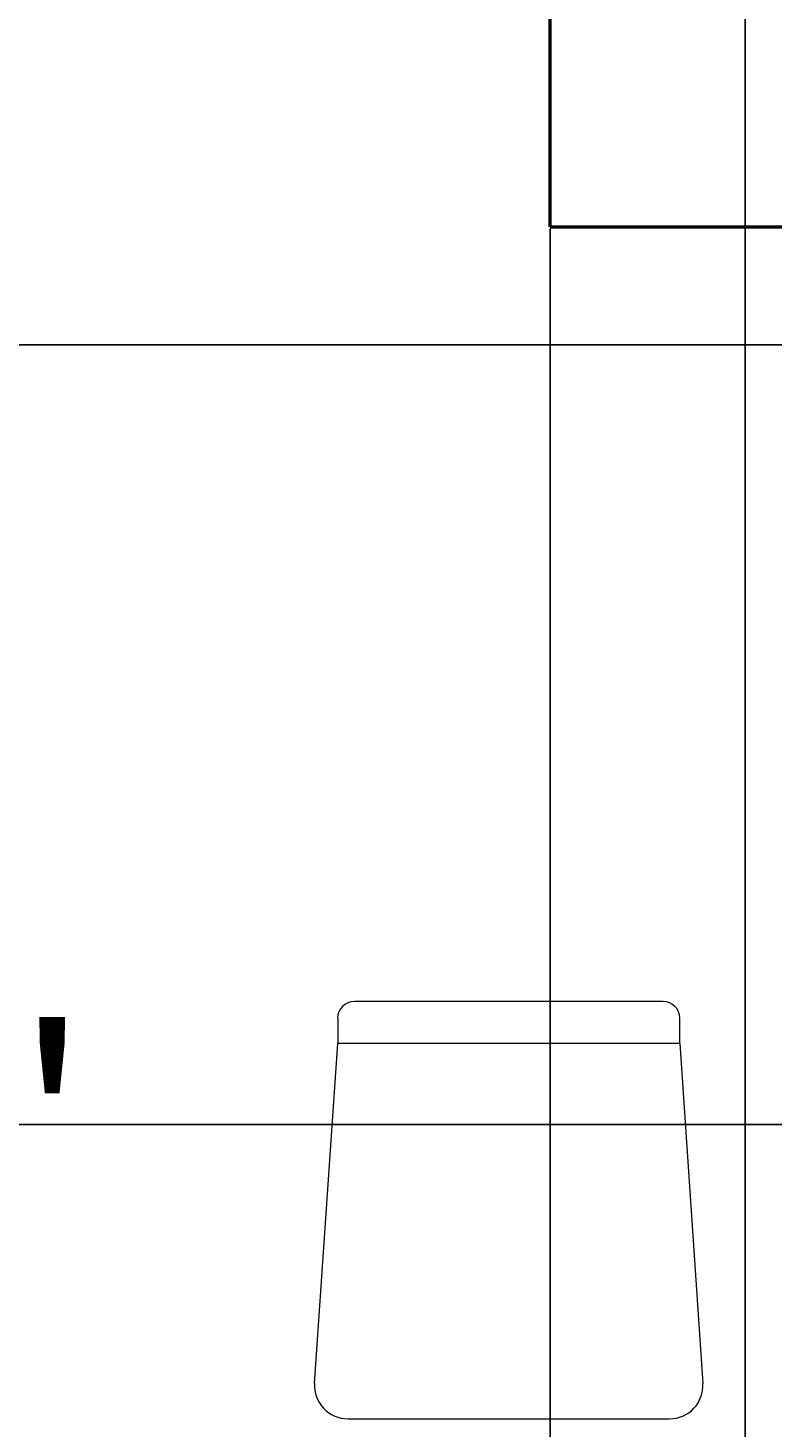
# Model space of a CAD drawing. Units: inches. Extents: x 0 to 281, y -535 to 46.
# Tile 9 of 22: x 173 to 196, y -168 to -125. Entities that reach past the tile are written whole.
import ezdxf

# ---------------------------------------------------------------- set-up
doc = ezdxf.new("R2010")
doc.units = ezdxf.units.IN
doc.header["$MEASUREMENT"] = 0
for name, color, linetype, lineweight in [('A-ANNO-DIMS', 2, 'Continuous', 18), ('A-FURN', 8, 'Continuous', 18), ('A-WALL', 7, 'Continuous', 50)]:
    doc.layers.add(name, color=color, linetype=linetype, lineweight=lineweight)
doc.styles.get("Standard").update_dxf_attribs({"font": 'arial.ttf'})
doc.dimstyles.get("Standard").update_dxf_attribs({"dimtxt": 0.18, "dimasz": 0.18, "dimexe": 0.18, "dimexo": 0.0625, "dimgap": 0.09, "dimtad": 0, "dimtih": 1, "dimtoh": 1, "dimdec": 0, "dimzin": 0, "dimdsep": 46, "dimlunit": 3, "dimtxsty": 'Standard', "dimcen": 0.09, "dimadec": 0, "dimazin": 0, "dimtfac": 1, "dimtdec": 0, "dimtofl": 0, "dimtmove": 0, "dimatfit": 3, "dimfxl": 1, "dimtolj": 1, "dimtzin": 0, "dimarcsym": 0})

# ---------------------------------------------------------------- blocks, each defined once
blk = doc.blocks.new('*D5')
at = {"layer": 'A-ANNO-DIMS', "color": 0, "lineweight": -2, "transparency": 16777216}
for p, q in [((93.459, -158.989), (93.459, -158.871)), ((93.639, -159.051), (153.846, -159.051)), ((234.279, -159.051), (174.072, -159.051)), ((234.459, -158.989), (234.459, -158.871))]:
    blk.add_line(p, q, dxfattribs=at)
at = {"layer": 'A-ANNO-DIMS', "color": 0, "transparency": 16777216}
for points in [[(93.639, -159.021), (93.639, -159.081), (93.459, -159.051)], [(234.279, -159.021), (234.279, -159.081), (234.459, -159.051)]]:
    blk.add_solid(points, dxfattribs=at)
at = {"layer": 'Defpoints', "color": 0, "transparency": 16777216}
for p in [(93.459, -159.051), (234.459, -159.051), (234.459, -159.051)]:
    blk.add_point(p, dxfattribs=at)
at = {"layer": 'A-ANNO-DIMS', "color": 0, "transparency": 16777216, "insert": (163.959, -159.051), "char_height": 6, "attachment_point": 5}
blk.add_mtext('\\A1;11\'-9"', dxfattribs=at)
blk = doc.blocks.new('CHAIR-DINING')
for p, q in [((10.729, 12.842), (1.225, 12.842)), ((0.712, 12.329), (0.712, 11.558)), ((11.243, 11.558), (11.243, 12.329)), ((0, 1.083), (0.712, 11.558)), ((11.243, 11.558), (0.712, 11.558)), ((11.243, 11.558), (11.954, 1.083)), ((1.026, 0), (10.928, 0))]:
    blk.add_line(p, q)
for centre, radius, start, end in [((1.225, 12.329), 0.514, 90, 180), ((10.729, 12.329), 0.514, 0, 90), ((1.026, 1.027), 1.027, 176.8779, 270), ((10.928, 1.027), 1.027, 270, 3.1221)]:
    blk.add_arc(centre, radius, start, end)
blk = doc.blocks.new('*D42')
at = {"layer": 'A-ANNO-DIMS', "color": 0, "lineweight": -2, "transparency": 16777216}
for p, q in [((165.459, -131.473), (165.459, -535.041)), ((189.459, -131.473), (189.459, -535.041)), ((165.639, -534.861), (177.128, -534.861)), ((189.279, -534.861), (177.79, -534.861))]:
    blk.add_line(p, q, dxfattribs=at)
at = {"layer": 'A-ANNO-DIMS', "color": 0, "transparency": 16777216}
for points in [[(165.639, -534.831), (165.639, -534.891), (165.459, -534.861)], [(189.279, -534.831), (189.279, -534.891), (189.459, -534.861)]]:
    blk.add_solid(points, dxfattribs=at)
at = {"layer": 'Defpoints', "color": 0, "transparency": 16777216}
for p in [(165.459, -131.411), (189.459, -131.411), (189.459, -534.861)]:
    blk.add_point(p, dxfattribs=at)
at = {"layer": 'A-ANNO-DIMS', "color": 0, "transparency": 16777216, "insert": (177.459, -534.861), "char_height": 0.18, "attachment_point": 5}
blk.add_mtext('\\A1;2\'-0"', dxfattribs=at)
blk = doc.blocks.new('*D43')
at = {"layer": 'A-ANNO-DIMS', "color": 0, "lineweight": -2, "transparency": 16777216}
for p, q in [((93.521, -135.051), (271.089, -135.051)), ((270.909, -135.231), (270.909, -146.869)), ((270.909, -158.871), (270.909, -147.233)), ((93.521, -159.051), (271.089, -159.051))]:
    blk.add_line(p, q, dxfattribs=at)
at = {"layer": 'A-ANNO-DIMS', "color": 0, "transparency": 16777216}
for points in [[(270.879, -135.231), (270.939, -135.231), (270.909, -135.051)], [(270.879, -158.871), (270.939, -158.871), (270.909, -159.051)]]:
    blk.add_solid(points, dxfattribs=at)
at = {"layer": 'Defpoints', "color": 0, "transparency": 16777216}
for p in [(93.459, -135.051), (93.459, -159.051), (270.909, -159.051)]:
    blk.add_point(p, dxfattribs=at)
at = {"layer": 'A-ANNO-DIMS', "color": 0, "transparency": 16777216, "insert": (270.909, -147.051), "char_height": 0.18, "attachment_point": 5}
blk.add_mtext('\\A1;2\'-0"', dxfattribs=at)
blk = doc.blocks.new('*D46')
at = {"layer": 'A-ANNO-DIMS', "color": 0, "lineweight": -2, "transparency": 16777216}
for p, q in [((159.459, -263.348), (159.459, 46.219)), ((195.459, -263.348), (195.459, 46.219)), ((159.639, 46.039), (177.13, 46.039)), ((195.279, 46.039), (177.788, 46.039))]:
    blk.add_line(p, q, dxfattribs=at)
at = {"layer": 'A-ANNO-DIMS', "color": 0, "transparency": 16777216}
for points in [[(159.639, 46.069), (159.639, 46.009), (159.459, 46.039)], [(195.279, 46.069), (195.279, 46.009), (195.459, 46.039)]]:
    blk.add_solid(points, dxfattribs=at)
at = {"layer": 'Defpoints', "color": 0, "transparency": 16777216}
for p in [(195.459, 46.039), (159.459, -263.411), (195.459, -263.411)]:
    blk.add_point(p, dxfattribs=at)
at = {"layer": 'A-ANNO-DIMS', "color": 0, "transparency": 16777216, "insert": (177.459, 46.039), "char_height": 0.18, "attachment_point": 5}
blk.add_mtext('\\A1;3\'-0"', dxfattribs=at)
blk = doc.blocks.new('*D48')
at = {"layer": 'A-ANNO-DIMS', "color": 0, "lineweight": -2, "transparency": 16777216}
for p, q in [((159.459, -392.348), (159.459, 46.219)), ((195.459, -392.348), (195.459, 46.219)), ((159.639, 46.039), (177.13, 46.039)), ((195.279, 46.039), (177.788, 46.039))]:
    blk.add_line(p, q, dxfattribs=at)
at = {"layer": 'A-ANNO-DIMS', "color": 0, "transparency": 16777216}
for points in [[(159.639, 46.069), (159.639, 46.009), (159.459, 46.039)], [(195.279, 46.069), (195.279, 46.009), (195.459, 46.039)]]:
    blk.add_solid(points, dxfattribs=at)
at = {"layer": 'Defpoints', "color": 0, "transparency": 16777216}
for p in [(195.459, 46.039), (159.459, -392.411), (195.459, -392.411)]:
    blk.add_point(p, dxfattribs=at)
at = {"layer": 'A-ANNO-DIMS', "color": 0, "transparency": 16777216, "insert": (177.459, 46.039), "char_height": 0.18, "attachment_point": 5}
blk.add_mtext('\\A1;3\'-0"', dxfattribs=at)

msp = doc.modelspace()

# ---------------------------------------------------------------- linework, layer by layer
at = {"layer": 'A-WALL'}
for q in [(189.459, -122.411), (243.459, -131.411)]:
    msp.add_line((189.459, -131.411), q, dxfattribs=at)

# ---------------------------------------------------------------- block references
at = {"layer": 'A-FURN'}
msp.add_blockref('CHAIR-DINING', (182.203, -168.111), dxfattribs=at)

# ---------------------------------------------------------------- dimensions: what is measured, and where the dimension line sits
at = {"layer": 'A-ANNO-DIMS'}
for base, p1, p2, override, picture, middle in [((195.459, 46.039), (159.459, -263.411), (195.459, -263.411), {"dimdec": 1, "dimlfac": 1, "dimrnd": 0, "dimzin": 1, "dimdsep": 46, "dimlunit": 4, "dimfrac": 2}, '*D46', (177.459, 46.039)), ((195.459, 46.039), (159.459, -392.411), (195.459, -392.411), {"dimdec": 1, "dimlfac": 1, "dimrnd": 0, "dimzin": 1, "dimdsep": 46, "dimlunit": 4, "dimfrac": 2}, '*D48', (177.459, 46.039)), ((189.459, -534.861), (165.459, -131.411), (189.459, -131.411), {"dimdec": 1, "dimlfac": 1, "dimrnd": 0, "dimzin": 1, "dimdsep": 46, "dimlunit": 4, "dimfrac": 2}, '*D42', (177.459, -534.861)), ((234.459, -159.051), (93.459, -159.051), (234.459, -159.051), {"dimtxt": 6, "dimclrd": 0, "dimclre": 0, "dimclrt": 0}, '*D5', (163.959, -159.051))]:
    dim = msp.add_linear_dim(base=base, p1=p1, p2=p2, dimstyle='Standard', override=override, dxfattribs=at)
    dim.commit()
    dim.dimension.update_dxf_attribs({"geometry": picture, "text_midpoint": middle})
dim = msp.add_linear_dim(base=(270.909, -159.051), p1=(93.459, -135.051), p2=(93.459, -159.051), angle=90, dimstyle='Standard', override={"dimdec": 1, "dimlfac": 1, "dimrnd": 0, "dimzin": 1, "dimdsep": 46, "dimlunit": 4, "dimfrac": 2}, dxfattribs=at)
dim.commit()
dim.dimension.update_dxf_attribs({"geometry": '*D43', "text_midpoint": (270.909, -147.051)})

doc.saveas('drawing.dxf')
